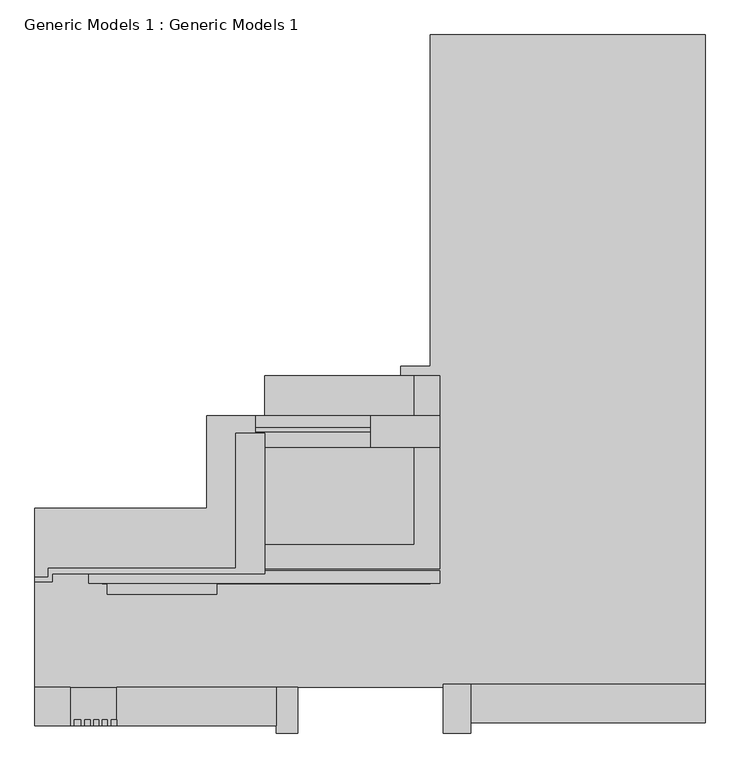
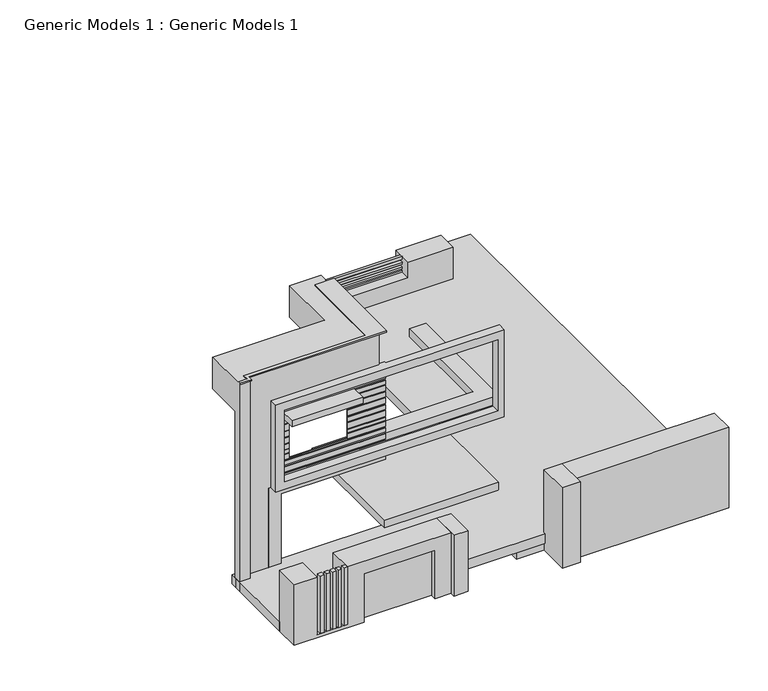
"""IFC4 building model written with IfcOpenShell, lengths in millimetres: proxy geometry, Generic Models 1 : Generic Models 1."""

from ifc_helpers import new_model, si_unit, frame, origin, place, context, project, spatial, polyline, outline, extrude, faceted_brep, source, transform, mapped, element, save


def generic_models_1_generic_models_1_c55d1f28(model_context):
    return source(origin(), model_context, "Body", "SolidModel", [
        extrude(outline(polyline([(-16089.4291921, -16199.7629514), (-16241.8291921, -16199.7629514), (-16241.8291921, -16047.3629514), (-16089.4291921, -16047.3629514), (-16089.4291921, -16199.7629514)])), frame((0.0, 0.0, -227.0298551), z_axis=(0.0, 0.0, 1.0), x_axis=(1.0, 0.0, 0.0)), (0.0, 0.0, 1.0), 2214.1363216),
        extrude(outline(polyline([(-15864.8371565, -16199.7629514), (-15998.1289156, -16199.7629514), (-15998.1289156, -16047.3629514), (-15864.8371565, -16047.3629514), (-15864.8371565, -16199.7629514)])), frame((0.0, 0.0, -227.0298551), z_axis=(0.0, 0.0, 1.0), x_axis=(1.0, 0.0, 0.0)), (0.0, 0.0, 1.0), 2214.1363216),
        extrude(outline(polyline([(-15659.2905319, -16199.7629514), (-15788.508411, -16199.7629514), (-15788.508411, -16047.3629514), (-15659.2905319, -16047.3629514), (-15659.2905319, -16199.7629514)])), frame((0.0, 0.0, -227.0298551), z_axis=(0.0, 0.0, 1.0), x_axis=(1.0, 0.0, 0.0)), (0.0, 0.0, 1.0), 2214.1363216),
        extrude(outline(polyline([(-15465.8233323, -16199.7629514), (-15585.534445, -16199.7629514), (-15585.534445, -16047.3629514), (-15465.8233323, -16047.3629514), (-15465.8233323, -16199.7629514)])), frame((0.0, 0.0, -227.0298551), z_axis=(0.0, 0.0, 1.0), x_axis=(1.0, 0.0, 0.0)), (0.0, 0.0, 1.0), 2214.1363216),
        extrude(outline(polyline([(-15235.287855, -16199.7629514), (-15369.2955938, -16199.7629514), (-15369.2955938, -16047.3629514), (-15235.287855, -16047.3629514), (-15235.287855, -16199.7629514)])), frame((0.0, 0.0, -227.0298551), z_axis=(0.0, 0.0, 1.0), x_axis=(1.0, 0.0, 0.0)), (0.0, 0.0, 1.0), 2214.1363216),
        faceted_brep([(-11456.7078521, -16199.7629514, -355.6), (-11456.7078521, -16199.7629514, 1987.1064665), (-15235.287855, -16199.7629514, 1987.1064665), (-15235.287855, -16199.7629514, -227.0298551), (-16341.728967, -16199.7629514, -227.0298551), (-16341.728967, -16199.7629514, 1987.1064665), (-17178.387855, -16199.7629514, 1987.1064665), (-17178.387855, -16199.7629514, -355.6), (-14630.1350928, -16199.7629514, -355.6), (-14630.1350928, -16199.7629514, 1517.5097908), (-12039.3350928, -16199.7629514, 1517.5097908), (-12039.3350928, -16199.7629514, -355.6), (-11456.7078521, -15285.3629514, -355.6), (-17178.387855, -15285.3629514, -355.6), (-17178.387855, -15285.3629514, 1987.1064665), (-16341.728967, -15285.3629514, 1987.1064665), (-16341.728967, -15285.3629514, -227.0298551), (-15235.287855, -15285.3629514, -227.0298551), (-15235.287855, -15285.3629514, 1987.1064665), (-11456.7078521, -15285.3629514, 1987.1064665), (-12039.3350928, -15971.1629514, -355.6), (-14630.1350928, -15971.1629514, -355.6), (-12039.3350928, -15971.1629514, 1517.5097908), (-14630.1350928, -15971.1629514, 1517.5097908)], [[[0, 1, 2, 3, 4, 5, 6, 7, 8, 9, 10, 11]], [[12, 13, 14, 15, 16, 17, 18, 19]], [[1, 0, 12, 19]], [[1, 19, 18, 2]], [[14, 6, 5, 15]], [[7, 6, 14, 13]], [[13, 12, 0, 11, 20, 21, 8, 7]], [[22, 23, 21, 20]], [[22, 20, 11, 10]], [[21, 23, 9, 8]], [[23, 22, 10, 9]], [[17, 3, 2, 18]], [[3, 17, 16, 4]], [[4, 16, 15, 5]]]),
        extrude(outline(polyline([(-6849.3388172, -16368.3651817), (-7500.3968742, -16368.3651817), (-7500.3968742, -15210.5768247), (-6849.3388172, -15210.5768247), (-6849.3388172, -16368.3651817)])), frame((0.0, 0.0, -660.4), z_axis=(0.0, 0.0, 1.0), x_axis=(1.0, 0.0, 0.0)), (0.0, 0.0, 1.0), 3094.2714904),
        extrude(outline(polyline([(-10941.984614, -16368.3651817), (-11456.7078521, -16368.3651817), (-11456.7078521, -15285.3629514), (-10941.984614, -15285.3629514), (-10941.984614, -16368.3651817)])), frame((0.0, 0.0, -355.6), z_axis=(0.0, 0.0, 1.0), x_axis=(1.0, 0.0, 0.0)), (0.0, 0.0, 1.0), 2342.7064665),
        extrude(outline(polyline([(-1290.687855, -16124.9768247), (-6849.3388172, -16124.9768247), (-6849.3388172, -15210.5768247), (-1290.687855, -15210.5768247), (-1290.687855, -16124.9768247)])), frame((0.0, 0.0, -660.4), z_axis=(0.0, 0.0, 1.0), x_axis=(1.0, 0.0, 0.0)), (0.0, 0.0, 1.0), 3094.2714904),
        extrude(outline(polyline([(0.0, -15996.8364088), (0.0, -15530.1363529), (2686.8964372, -15530.1363529), (2686.8964372, -11730.087855), (3048.0, -11730.087855), (3048.0, -15996.8364088), (0.0, -15996.8364088)])), frame((0.0, -12518.1768247, 0.0), z_axis=(0.0, 1.0, 0.0), x_axis=(0.0, 0.0, 1.0)), (0.0, 0.0, 1.0), 50.8),
        faceted_brep([(-12870.8892671, -12467.3768247, 5799.0532246), (-15461.6892671, -12467.3768247, 5799.0532246), (-15461.6892671, -13076.9768247, 5799.0532246), (-12870.8892671, -13076.9768247, 5799.0532246), (-12870.8892671, -12518.1768247, 5799.0532246), (-12870.8892671, -12492.7768247, 5799.0532246), (-12870.8892671, -13076.9768247, 5570.4532246), (-15461.6892671, -13076.9768247, 5570.4532246), (-15461.6892671, -12518.1768247, 5570.4532246), (-15461.6892671, -12492.7768247, 5570.4532246), (-15461.6892671, -12467.3768247, 5570.4532246), (-12870.8892671, -12467.3768247, 5570.4532246), (-12870.8892671, -12492.7768247, 5570.4532246), (-12870.8892671, -12518.1768247, 5570.4532246)], [[[0, 1, 2, 3, 4, 5]], [[6, 7, 8, 9, 10, 11, 12, 13]], [[2, 1, 10, 9, 8, 7]], [[3, 2, 7, 6]], [[11, 0, 5, 4, 3, 6, 13, 12]], [[1, 0, 11, 10]]]),
        faceted_brep([(-15461.6892671, -12518.1768247, 5570.4532246), (-15461.6892671, -12518.1768247, 5730.3391242), (-13101.687855, -12518.1768247, 5730.3391242), (-13101.687855, -12518.1768247, 5570.4532246), (-11730.087855, -12518.1768247, 5570.4532246), (-11730.087855, -12518.1768247, 5728.2702716), (-12870.8892671, -12518.1768247, 5728.2702716), (-12870.8892671, -12518.1768247, 5799.0532246), (-11730.087855, -12518.1768247, 5799.0532246), (-11730.087855, -12518.1768247, 5884.5214024), (-15586.1498871, -12518.1768247, 5884.5214024), (-15586.1498871, -12518.1768247, 5570.4532246), (-11730.087855, -12518.1768247, 6096.0), (-15586.1498871, -12518.1768247, 6096.0), (-15586.1498871, -12518.1768247, 5970.3790497), (-11730.087855, -12518.1768247, 5970.3790497), (-15586.1498871, -12518.1768247, 3352.8), (-11730.087855, -12518.1768247, 3352.8), (-11730.087855, -12518.1768247, 3412.5091158), (-15586.1498871, -12518.1768247, 3412.5091158), (-15901.1547186, -12518.1768247, 3048.0), (-15901.1547186, -12518.1768247, 6400.8), (-11958.687855, -12518.1768247, 6400.8), (-11958.687855, -12518.1768247, 7620.0), (-16788.8398722, -12518.1768247, 7620.0), (-16788.8398722, -12518.1768247, 0.0), (-15996.8364088, -12518.1768247, 0.0), (-15996.8364088, -12518.1768247, 3048.0), (-15235.287855, -12518.1768247, 5327.0826559), (-15235.287855, -12518.1768247, 5538.7343996), (-15586.1498871, -12518.1768247, 5538.7343996), (-15586.1498871, -12518.1768247, 5327.0826559), (-15235.287855, -12518.1768247, 5044.9109534), (-15235.287855, -12518.1768247, 5287.7922483), (-15586.1498871, -12518.1768247, 5287.7922483), (-15586.1498871, -12518.1768247, 5044.9109534), (-15235.287855, -12518.1768247, 4811.6817974), (-15235.287855, -12518.1768247, 5016.4973729), (-15586.1498871, -12518.1768247, 5016.4973729), (-15586.1498871, -12518.1768247, 4811.6817974), (-15235.287855, -12518.1768247, 4555.1170493), (-15235.287855, -12518.1768247, 4781.5044787), (-15586.1498871, -12518.1768247, 4781.5044787), (-15586.1498871, -12518.1768247, 4555.1170493), (-15235.287855, -12518.1768247, 4336.7848119), (-15235.287855, -12518.1768247, 4514.0666896), (-15586.1498871, -12518.1768247, 4514.0666896), (-15586.1498871, -12518.1768247, 4336.7848119), (-15235.287855, -12518.1768247, 3946.5178454), (-15235.287855, -12518.1768247, 4137.641103), (-15586.1498871, -12518.1768247, 4137.641103), (-15586.1498871, -12518.1768247, 3946.5178454), (-15235.287855, -12518.1768247, 4166.0944084), (-15235.287855, -12518.1768247, 4310.9475995), (-15586.1498871, -12518.1768247, 4310.9475995), (-15586.1498871, -12518.1768247, 4166.0944084), (-13101.687855, -12518.1768247, 5522.4550301), (-13101.687855, -12518.1768247, 5326.9611332), (-11730.087855, -12518.1768247, 5326.9611332), (-11730.087855, -12518.1768247, 5522.4550301), (-13101.687855, -12518.1768247, 5287.7922483), (-13101.687855, -12518.1768247, 5085.9613131), (-11730.087855, -12518.1768247, 5085.9613131), (-11730.087855, -12518.1768247, 5287.7922483), (-13101.687855, -12518.1768247, 5044.9109534), (-13101.687855, -12518.1768247, 4838.4284848), (-11730.087855, -12518.1768247, 4838.4284848), (-11730.087855, -12518.1768247, 5044.9109534), (-13101.687855, -12518.1768247, 4781.5044787), (-13101.687855, -12518.1768247, 4610.4613132), (-11730.087855, -12518.1768247, 4610.4613132), (-11730.087855, -12518.1768247, 4781.5044787), (-13101.687855, -12518.1768247, 4572.0), (-13101.687855, -12518.1768247, 4336.7848119), (-11730.087855, -12518.1768247, 4336.7848119), (-11730.087855, -12518.1768247, 4572.0), (-13101.687855, -12518.1768247, 4145.9759566), (-13101.687855, -12518.1768247, 3946.5178454), (-11730.087855, -12518.1768247, 3946.5178454), (-11730.087855, -12518.1768247, 4145.9759566), (-13101.687855, -12518.1768247, 4295.7344522), (-13101.687855, -12518.1768247, 4172.0616915), (-11730.087855, -12518.1768247, 4172.0616915), (-11730.087855, -12518.1768247, 4295.7344522), (-15586.1498871, -12518.1768247, 3901.5625647), (-15586.1498871, -12518.1768247, 3730.5193993), (-11730.087855, -12518.1768247, 3730.5193993), (-11730.087855, -12518.1768247, 3901.5625647), (-15586.1498871, -12518.1768247, 3657.6), (-15586.1498871, -12518.1768247, 3460.7849638), (-11730.087855, -12518.1768247, 3460.7849638), (-11730.087855, -12518.1768247, 3657.6), (-11730.087855, -12467.3768247, 6400.8), (-11730.087855, -12467.3768247, 3048.0), (-15996.8364088, -12467.3768247, 3048.0), (-15996.8364088, -12467.3768247, 0.0), (-17178.387855, -12467.3768247, 0.0), (-17178.387855, -12467.3768247, 6400.8), (-11958.687855, -12467.3768247, 6400.8), (-15235.287855, -12467.3768247, 5570.4532246), (-15235.287855, -12467.3768247, 3946.5178454), (-13101.687855, -12467.3768247, 3946.5178454), (-13101.687855, -12467.3768247, 5730.3391242), (-15461.6892671, -12467.3768247, 5730.3391242), (-15461.6892671, -12467.3768247, 5570.4532246), (-11730.087855, -12518.1768247, 6400.8), (-11730.087855, -12492.7768247, 5970.3790497), (-11730.087855, -12492.7768247, 5884.5214024), (-11730.087855, -12492.7768247, 5799.0532246), (-11730.087855, -12492.7768247, 5728.2702716), (-11730.087855, -12492.7768247, 5570.4532246), (-11730.087855, -12492.7768247, 5522.4550301), (-11730.087855, -12492.7768247, 5326.9611332), (-11730.087855, -12492.7768247, 5287.7922483), (-11730.087855, -12492.7768247, 5085.9613131), (-11730.087855, -12492.7768247, 5044.9109534), (-11730.087855, -12492.7768247, 4838.4284848), (-11730.087855, -12492.7768247, 4781.5044787), (-11730.087855, -12492.7768247, 4610.4613132), (-11730.087855, -12492.7768247, 4572.0), (-11730.087855, -12492.7768247, 4336.7848119), (-11730.087855, -12492.7768247, 4295.7344522), (-11730.087855, -12492.7768247, 4172.0616915), (-11730.087855, -12492.7768247, 4145.9759566), (-11730.087855, -12492.7768247, 3946.5178454), (-11730.087855, -12492.7768247, 3901.5625647), (-11730.087855, -12492.7768247, 3730.5193993), (-11730.087855, -12492.7768247, 3657.6), (-11730.087855, -12492.7768247, 3460.7849638), (-11730.087855, -12492.7768247, 3412.5091158), (-11730.087855, -12518.1768247, 3048.0), (-17178.387855, -11041.464427, 7620.0), (-17178.387855, -11041.464427, 6400.8), (-17178.387855, -12518.1768247, 0.0), (-17178.387855, -12518.1768247, -355.6), (-17178.387855, -12746.7768247, -355.6), (-17178.387855, -12746.7768247, 7620.0), (-17178.387855, -12784.9186062, 7620.0), (-17178.387855, -12784.9186062, 7670.8), (-17178.387855, -12670.135159, 7670.8), (-17178.387855, -12670.135159, 7620.0), (-15901.1547186, -12822.9768247, 6400.8), (-7577.187855, -12822.9768247, 6400.8), (-7577.187855, -12518.1768247, 6400.8), (-7577.187855, -12518.1768247, 3048.0), (-7805.787855, -12518.1768247, 3352.8), (-7805.787855, -12518.1768247, 6096.0), (-7805.787855, -12822.9768247, 6096.0), (-15586.1498871, -12822.9768247, 6096.0), (-7577.187855, -12822.9768247, 3048.0), (-15586.1498871, -12822.9768247, 3352.8), (-15586.1498871, -12492.7768247, 3412.5091158), (-15586.1498871, -12492.7768247, 3460.7849638), (-15586.1498871, -12492.7768247, 3657.6), (-15586.1498871, -12492.7768247, 3730.5193993), (-15586.1498871, -12492.7768247, 3901.5625647), (-15586.1498871, -12492.7768247, 3946.5178454), (-15586.1498871, -12492.7768247, 4137.641103), (-15586.1498871, -12492.7768247, 4166.0944084), (-15586.1498871, -12492.7768247, 4310.9475995), (-15586.1498871, -12492.7768247, 4336.7848119), (-15586.1498871, -12492.7768247, 4514.0666896), (-15586.1498871, -12492.7768247, 4555.1170493), (-15586.1498871, -12492.7768247, 4781.5044787), (-15586.1498871, -12492.7768247, 4811.6817974), (-15586.1498871, -12492.7768247, 5016.4973729), (-15586.1498871, -12492.7768247, 5044.9109534), (-15586.1498871, -12492.7768247, 5287.7922483), (-15586.1498871, -12492.7768247, 5327.0826559), (-15586.1498871, -12492.7768247, 5538.7343996), (-15586.1498871, -12492.7768247, 5570.4532246), (-15586.1498871, -12492.7768247, 5884.5214024), (-15586.1498871, -12492.7768247, 5970.3790497), (-15901.1547186, -12822.9768247, 3048.0), (-13101.687855, -12492.7768247, 3946.5178454), (-13101.687855, -12492.7768247, 4145.9759566), (-13101.687855, -12492.7768247, 4172.0616915), (-13101.687855, -12492.7768247, 4295.7344522), (-13101.687855, -12492.7768247, 4336.7848119), (-13101.687855, -12492.7768247, 4572.0), (-13101.687855, -12492.7768247, 4610.4613132), (-13101.687855, -12492.7768247, 4781.5044787), (-13101.687855, -12492.7768247, 4838.4284848), (-13101.687855, -12492.7768247, 5044.9109534), (-13101.687855, -12492.7768247, 5085.9613131), (-13101.687855, -12492.7768247, 5287.7922483), (-13101.687855, -12492.7768247, 5326.9611332), (-13101.687855, -12492.7768247, 5522.4550301), (-13101.687855, -12492.7768247, 5570.4532246), (-15235.287855, -12492.7768247, 3946.5178454), (-15235.287855, -12492.7768247, 5570.4532246), (-15235.287855, -12492.7768247, 5538.7343996), (-15235.287855, -12492.7768247, 5327.0826559), (-15235.287855, -12492.7768247, 5287.7922483), (-15235.287855, -12492.7768247, 5044.9109534), (-15235.287855, -12492.7768247, 5016.4973729), (-15235.287855, -12492.7768247, 4811.6817974), (-15235.287855, -12492.7768247, 4781.5044787), (-15235.287855, -12492.7768247, 4555.1170493), (-15235.287855, -12492.7768247, 4514.0666896), (-15235.287855, -12492.7768247, 4336.7848119), (-15235.287855, -12492.7768247, 4310.9475995), (-15235.287855, -12492.7768247, 4166.0944084), (-15235.287855, -12492.7768247, 4137.641103), (-15461.6892671, -12492.7768247, 5570.4532246), (-7805.787855, -12822.9768247, 3352.8), (-7577.187855, -9596.8215151, 7620.0), (-7577.187855, -8847.8768247, 7620.0), (-9215.487855, -8847.8768247, 7620.0), (-9215.487855, -9596.8215151, 7620.0), (-13101.687855, -8847.8768247, 7620.0), (-13101.687855, -11041.464427, 7620.0), (-16865.0398722, -12670.135159, 7620.0), (-16865.0398722, -12466.935159, 7620.0), (-16764.7547186, -12466.935159, 7620.0), (-16764.7547186, -12467.3768247, 7620.0), (-12415.887855, -12467.3768247, 7620.0), (-12415.887855, -9266.9768247, 7620.0), (-11958.687855, -9266.9768247, 7620.0), (-11958.687855, -8847.8768247, 7620.0), (-13101.687855, -11041.464427, 6400.8), (-13101.687855, -8847.8768247, 6400.8), (-7577.187855, -8847.8768247, 6400.8), (-7577.187855, -9596.8215151, 6400.8), (-11958.687855, -9596.8215151, 6400.8), (-11958.687855, -9596.8215151, 7010.4), (-11958.687855, -8847.8768247, 7010.4), (-9215.487855, -8847.8768247, 7010.4), (-9215.487855, -9596.8215151, 7010.4), (-16788.8398722, -12746.7768247, -355.6), (-16788.8398722, -12746.7768247, 7620.0), (-16788.8398722, -12518.1768247, -355.6), (-16865.0398722, -12670.135159, 7670.8), (-16764.7547186, -12784.9186062, 7670.8), (-16764.7547186, -12784.9186062, 7620.0), (-16764.7547186, -12466.935159, 7670.8), (-16764.7547186, -12467.3768247, 7670.8), (-16764.7547186, -12593.5702046, 7620.0), (-16764.7547186, -12593.5702046, 7670.8), (-16865.0398722, -12466.935159, 7670.8), (-11730.087855, -12593.5702046, 7670.8), (-11730.087855, -9266.9768247, 7670.8), (-12415.887855, -9266.9768247, 7670.8), (-12415.887855, -12467.3768247, 7670.8), (-11730.087855, -12593.5702046, 7620.0), (-11730.087855, -9266.9768247, 7620.0), (-12870.8892671, -12492.7768247, 5799.0532246), (-12870.8892671, -12492.7768247, 5728.2702716)], [[[0, 1, 2, 3, 4, 5, 6, 7, 8, 9, 10, 11]], [[12, 13, 14, 15]], [[16, 17, 18, 19]], [[20, 21, 22, 23, 24, 25, 26, 27]], [[28, 29, 30, 31]], [[32, 33, 34, 35]], [[36, 37, 38, 39]], [[40, 41, 42, 43]], [[44, 45, 46, 47]], [[48, 49, 50, 51]], [[52, 53, 54, 55]], [[56, 57, 58, 59]], [[60, 61, 62, 63]], [[64, 65, 66, 67]], [[68, 69, 70, 71]], [[72, 73, 74, 75]], [[76, 77, 78, 79]], [[80, 81, 82, 83]], [[84, 85, 86, 87]], [[88, 89, 90, 91]], [[92, 93, 94, 95, 96, 97, 98], [99, 100, 101, 102, 103, 104]], [[92, 105, 12, 15, 106, 107, 9, 8, 108, 109, 5, 4, 110, 111, 59, 58, 112, 113, 63, 62, 114, 115, 67, 66, 116, 117, 71, 70, 118, 119, 75, 74, 120, 121, 83, 82, 122, 123, 79, 78, 124, 125, 87, 86, 126, 127, 91, 90, 128, 129, 18, 17, 130, 93]], [[131, 132, 97, 96, 133, 134, 135, 136, 137, 138, 139, 140]], [[105, 92, 98, 22, 21, 141, 142, 143]], [[12, 105, 143, 144, 130, 17, 145, 146]], [[13, 12, 146, 147, 148]], [[143, 142, 149, 144]], [[148, 150, 16, 19, 151, 152, 89, 88, 153, 154, 85, 84, 155, 156, 51, 50, 157, 158, 55, 54, 159, 160, 47, 46, 161, 162, 43, 42, 163, 164, 39, 38, 165, 166, 35, 34, 167, 168, 31, 30, 169, 170, 11, 10, 171, 172, 14, 13]], [[141, 21, 20, 173]], [[2, 102, 101, 174, 77, 76, 175, 176, 81, 80, 177, 178, 73, 72, 179, 180, 69, 68, 181, 182, 65, 64, 183, 184, 61, 60, 185, 186, 57, 56, 187, 188, 3]], [[101, 100, 189, 174]], [[100, 99, 190, 191, 29, 28, 192, 193, 33, 32, 194, 195, 37, 36, 196, 197, 41, 40, 198, 199, 45, 44, 200, 201, 53, 52, 202, 203, 49, 48, 189]], [[99, 104, 204, 190]], [[1, 0, 204, 104, 103]], [[1, 103, 102, 2]], [[93, 130, 144, 149, 173, 20, 27, 94]], [[17, 16, 150, 205, 145]], [[205, 147, 146, 145]], [[96, 95, 26, 25, 133]], [[27, 26, 95, 94]], [[206, 207, 208, 209]], [[210, 211, 131, 140, 212, 213, 214, 215, 216, 217, 218, 219]], [[97, 132, 220, 221, 222, 223, 224, 98]], [[23, 22, 98, 224, 225, 226, 219, 218]], [[132, 131, 211, 220]], [[221, 210, 219, 226, 227, 208, 207, 222]], [[211, 210, 221, 220]], [[207, 206, 223, 222]], [[224, 223, 206, 209, 228, 225]], [[136, 135, 229, 230]], [[231, 134, 133, 25]], [[229, 135, 134, 231]], [[230, 229, 231, 25, 24]], [[140, 139, 232, 212]], [[233, 138, 137, 234]], [[214, 235, 236, 215]], [[237, 238, 233, 234]], [[239, 235, 214, 213]], [[232, 239, 213, 212]], [[238, 240, 241, 242, 243, 236, 235, 239, 232, 139, 138, 233]], [[244, 237, 234, 137, 136, 230, 24, 23, 218, 245]], [[240, 244, 245, 241]], [[216, 215, 236, 243]], [[240, 238, 237, 244]], [[173, 149, 142, 141], [150, 148, 147, 205]], [[227, 228, 209, 208]], [[228, 227, 226, 225]], [[242, 241, 245, 218, 217]], [[243, 242, 217, 216]], [[156, 155, 125, 124, 174, 189]], [[170, 169, 191, 190, 204]], [[106, 172, 171, 107]], [[108, 246, 247, 109]], [[110, 188, 187, 111]], [[112, 186, 185, 113]], [[114, 184, 183, 115]], [[116, 182, 181, 117]], [[118, 180, 179, 119]], [[120, 178, 177, 121]], [[122, 176, 175, 123]], [[126, 154, 153, 127]], [[128, 152, 151, 129]], [[192, 168, 167, 193]], [[194, 166, 165, 195]], [[196, 164, 163, 197]], [[198, 162, 161, 199]], [[200, 160, 159, 201]], [[202, 158, 157, 203]], [[107, 171, 10, 9]], [[172, 106, 15, 14]], [[109, 247, 6, 5]], [[247, 246, 7, 6]], [[246, 108, 8, 7]], [[111, 187, 56, 59]], [[188, 110, 4, 3]], [[113, 185, 60, 63]], [[186, 112, 58, 57]], [[115, 183, 64, 67]], [[184, 114, 62, 61]], [[117, 181, 68, 71]], [[182, 116, 66, 65]], [[119, 179, 72, 75]], [[180, 118, 70, 69]], [[121, 177, 80, 83]], [[178, 120, 74, 73]], [[123, 175, 76, 79]], [[176, 122, 82, 81]], [[125, 155, 84, 87]], [[51, 156, 189, 48]], [[174, 124, 78, 77]], [[127, 153, 88, 91]], [[154, 126, 86, 85]], [[129, 151, 19, 18]], [[152, 128, 90, 89]], [[191, 169, 30, 29]], [[11, 170, 204, 0]], [[193, 167, 34, 33]], [[168, 192, 28, 31]], [[195, 165, 38, 37]], [[166, 194, 32, 35]], [[197, 163, 42, 41]], [[164, 196, 36, 39]], [[199, 161, 46, 45]], [[162, 198, 40, 43]], [[201, 159, 54, 53]], [[160, 200, 44, 47]], [[203, 157, 50, 49]], [[158, 202, 52, 55]]]),
        extrude(outline(polyline([(-11958.687855, -9230.9142381), (-11958.687855, -9129.3142381), (-9215.487855, -9129.3142381), (-9215.487855, -9230.9142381), (-11958.687855, -9230.9142381)])), frame((0.0, 0.0, 7518.4), z_axis=(0.0, 0.0, 1.0), x_axis=(1.0, 0.0, 0.0)), (0.0, 0.0, 1.0), 101.6),
        extrude(outline(polyline([(-11958.687855, -9230.9142381), (-11958.687855, -9129.3142381), (-9215.487855, -9129.3142381), (-9215.487855, -9230.9142381), (-11958.687855, -9230.9142381)])), frame((0.0, 0.0, 7312.5441915), z_axis=(0.0, 0.0, 1.0), x_axis=(1.0, 0.0, 0.0)), (0.0, 0.0, 1.0), 90.25082),
        extrude(outline(polyline([(-11958.687855, -9230.9142381), (-11958.687855, -9129.3142381), (-9215.487855, -9129.3142381), (-9215.487855, -9230.9142381), (-11958.687855, -9230.9142381)])), frame((0.0, 0.0, 7138.0694699), z_axis=(0.0, 0.0, 1.0), x_axis=(1.0, 0.0, 0.0)), (0.0, 0.0, 1.0), 85.855648),
        extrude(outline(polyline([(-11958.687855, -9222.3491699), (-11958.687855, -9129.3142381), (-9215.487855, -9129.3142381), (-9215.487855, -9222.3491699), (-11958.687855, -9222.3491699)])), frame((0.0, 0.0, 7010.4), z_axis=(0.0, 0.0, 1.0), x_axis=(1.0, 0.0, 0.0)), (0.0, 0.0, 1.0), 73.2664781),
        extrude(outline(polyline([(-7577.187855, -12467.3768247), (-11730.087855, -12467.3768247), (-11730.087855, -11906.0921671), (-8186.787855, -11906.0921671), (-8186.787855, -7895.3768247), (-7577.187855, -7895.3768247), (-7577.187855, -12467.3768247)])), frame((0.0, 0.0, 3352.8), z_axis=(0.0, 0.0, 1.0), x_axis=(1.0, 0.0, 0.0)), (0.0, 0.0, 1.0), 304.8),
        faceted_brep([(-7577.187855, -7895.3768247, 304.8), (-11730.087855, -7895.3768247, 304.8), (-11730.087855, -12467.3768247, 304.8), (-7577.187855, -12467.3768247, 304.8), (-11730.087855, -12280.2857433, 0.0), (-11730.087855, -7895.3768247, 0.0), (-8509.1233035, -7895.3768247, 0.0), (-8509.1233035, -12280.2857433, 0.0), (-7577.187855, -7895.3768247, 0.0), (-11730.087855, -12467.3768247, 0.0), (-7577.187855, -12467.3768247, 0.0), (-7805.787855, 181.8231753, -355.6), (-1290.687855, 181.8231753, -355.6), (-1290.687855, -7666.7768247, -355.6), (-7805.787855, -7666.7768247, -355.6), (-1290.687855, 181.8231753, 0.0), (-7805.787855, 181.8231753, 0.0), (-7805.787855, -7666.7768247, 0.0), (-8509.1233035, -7666.7768247, 0.0), (-17178.387855, -12280.2857433, 0.0), (-17178.387855, -15285.3629514, 0.0), (-7500.3968742, -15285.3629514, 0.0), (-7500.3968742, -15210.5768247, 0.0), (-1290.687855, -15210.5768247, 0.0), (-1290.687855, -15210.5768247, -660.4), (-1290.687855, -7666.7768247, -660.4), (-7500.3968742, -15285.3629514, -355.6), (-17178.387855, -15285.3629514, -355.6), (-17178.387855, -12280.2857433, -355.6), (-8509.1233035, -12280.2857433, -355.6), (-8509.1233035, -15210.5768247, -355.6), (-7500.3968742, -15210.5768247, -355.6), (-8509.1233035, -15210.5768247, -660.4), (-8509.1233035, -7666.7768247, -660.4)], [[[0, 1, 2, 3]], [[4, 5, 6, 7]], [[1, 0, 8, 6, 5]], [[2, 1, 5, 4, 9]], [[3, 2, 9, 10]], [[0, 3, 10, 8]], [[11, 12, 13, 14]], [[15, 16, 17, 18, 6, 8, 10, 9, 4, 19, 20, 21, 22, 23]], [[12, 11, 16, 15]], [[12, 15, 23, 24, 25, 13]], [[16, 11, 14, 17]], [[26, 27, 28, 29, 30, 31]], [[27, 26, 21, 20]], [[28, 27, 20, 19]], [[28, 19, 4, 7, 29]], [[21, 26, 31, 22]], [[25, 24, 32, 33]], [[32, 24, 23, 22, 31, 30]], [[33, 32, 30, 29, 7, 6, 18]], [[25, 33, 18, 17, 14, 13]]]),
    ])


if __name__ == "__main__":
    model = new_model("IFC4")
    model_context = context("Model", 3, world=origin())
    ifc_project = project(units=[si_unit("LENGTHUNIT", "METRE", prefix="MILLI")], contexts=[model_context])
    site = spatial("IfcSite", under=ifc_project)
    building = spatial("IfcBuilding", under=site)
    placement = place(None, origin())
    generic_models_1_generic_models_1_shape = generic_models_1_generic_models_1_c55d1f28(model_context)
    element("IfcBuildingElementProxy", 1, Name="Generic Models 1 : Generic Models 1", ObjectType="Generic Models 1 : Generic Models 1", at=placement, inside=building, context=model_context, shape_type="MappedRepresentation", body=[
        mapped(generic_models_1_generic_models_1_shape, transform((0.0, 0.0, 0.0), x_axis=(1.0, 0.0, 0.0), y_axis=(0.0, 1.0, 0.0), z_axis=(0.0, 0.0, 1.0))),
    ])
    save(model, "model.ifc")
